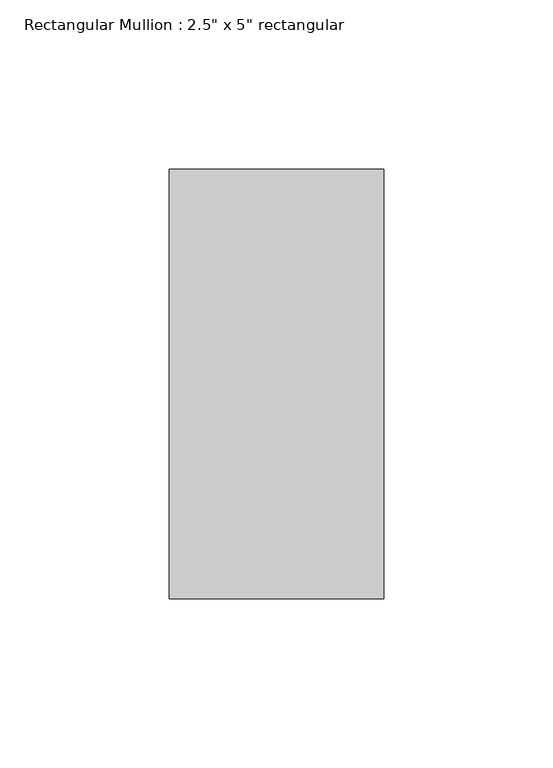
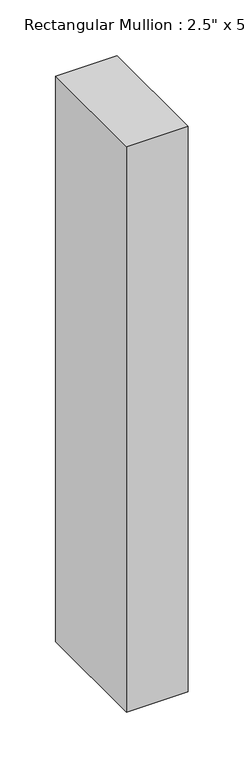
"""IFC4 building model written with IfcOpenShell, lengths in millimetres: member geometry."""

from ifc_helpers import new_model, si_unit, frame, origin, place, context, project, spatial, polyline, outline, extrude, source, transform, mapped, element, save


def member_c3a59c23(model_context):
    return source(origin(), model_context, "Body", "SweptSolid", [
        extrude(outline(polyline([(0.0, 63.5), (0.0, -63.5), (-63.5, -63.5), (-63.5, 63.5), (0.0, 63.5)])), frame((0.0, 0.0, -618.0666667), z_axis=(0.0, 0.0, 1.0), x_axis=(1.0, 0.0, 0.0)), (0.0, 0.0, 1.0), 618.0666667),
    ])


if __name__ == "__main__":
    model = new_model("IFC4")
    model_context = context("Model", 3, world=origin())
    ifc_project = project(units=[si_unit("LENGTHUNIT", "METRE", prefix="MILLI")], contexts=[model_context])
    site = spatial("IfcSite", under=ifc_project)
    building = spatial("IfcBuilding", under=site)
    placement = place(None, origin())
    member_shape = member_c3a59c23(model_context)
    element("IfcMember", 1, ObjectType="Rectangular Mullion : 2.5\" x 5\" rectangular", at=placement, inside=building, context=model_context, shape_type="MappedRepresentation", body=[
        mapped(member_shape, transform((0.0, 0.0, 0.0), x_axis=(1.0, 0.0, 0.0), y_axis=(0.0, 1.0, 0.0), z_axis=(0.0, 0.0, 1.0))),
    ])
    save(model, "model.ifc")

# Revit data of these elements
# Type "Rectangular Mullion : 2.5\" x 5\" rectangular"
#   built-in parameter 1007304 = 0.416667 (stored number, unit not read)
#   built-in parameter 1007301 = 0.104167 (stored number, unit not read)
#   built-in parameter 1007300 = 0.104167 (stored number, unit not read)
# Element 1 (IfcMember, "Rectangular Mullion : 2.5\" x 5\" rectangular")
#   Materials on its faces: "Door - Frame"
# Materials
#   "Door - Frame": colour RGB 118 70 51, transparency 0, Cost = 0
